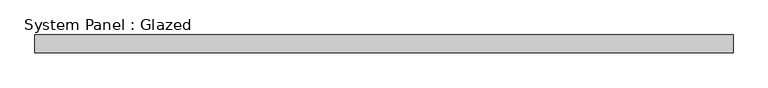
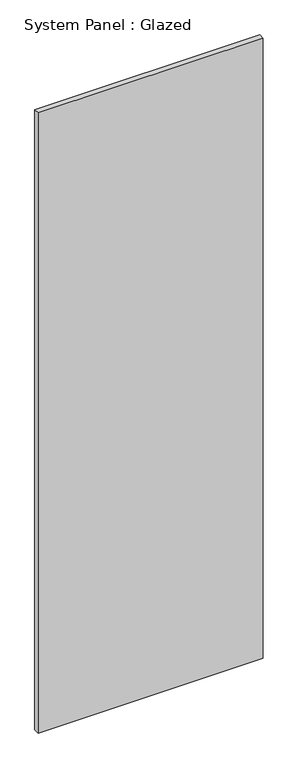
"""IFC4 building model written with IfcOpenShell, lengths in millimetres: plate geometry, System Panel : Glazed."""

from ifc_helpers import new_model, si_unit, origin, origin_with_axes, place, context, project, spatial, polyline, outline, extrude, source, transform, mapped, element, save


def system_panel_glazed_62014e10(model_context):
    return source(origin(), model_context, "Body", "SweptSolid", [
        extrude(outline(polyline([(501.65, 19.05), (-501.65, 19.05), (-501.65, 44.45), (501.65, 44.45), (501.65, 19.05)])), origin_with_axes(), (0.0, 0.0, 1.0), 2921.0),
    ])


if __name__ == "__main__":
    model = new_model("IFC4")
    model_context = context("Model", 3, world=origin())
    ifc_project = project(units=[si_unit("LENGTHUNIT", "METRE", prefix="MILLI")], contexts=[model_context])
    site = spatial("IfcSite", under=ifc_project)
    building = spatial("IfcBuilding", under=site)
    placement = place(None, origin())
    system_panel_glazed_shape = system_panel_glazed_62014e10(model_context)
    element("IfcPlate", 1, ObjectType="System Panel : Glazed", at=placement, inside=building, context=model_context, shape_type="MappedRepresentation", body=[
        mapped(system_panel_glazed_shape, transform((0.0, 0.0, 0.0), x_axis=(1.0, 0.0, 0.0), y_axis=(0.0, 1.0, 0.0), z_axis=(0.0, 0.0, 1.0))),
    ])
    save(model, "model.ifc")

# Revit data of these elements
# Type "System Panel : Glazed"
#   Construction Type Id = "GSP4R"
#   Analytic Construction = "1/8 in Pilkington single glazing"
#   Visual Light Transmittance = 0.9
#   Solar Heat Gain Coefficient = 0.86
#   Heat Transfer Coefficient (U) = 1.18115 BTU/(h·ft²·°F)
#   Define Thermal Properties by = 1
# Element 1 (IfcPlate, "System Panel : Glazed")
#   Materials on its faces: "Glass"
# Materials
#   "Glass": class "Glass", colour RGB 0 128 192, transparency 0.75, Description = "Soda Lime Glass", Cost = 0
